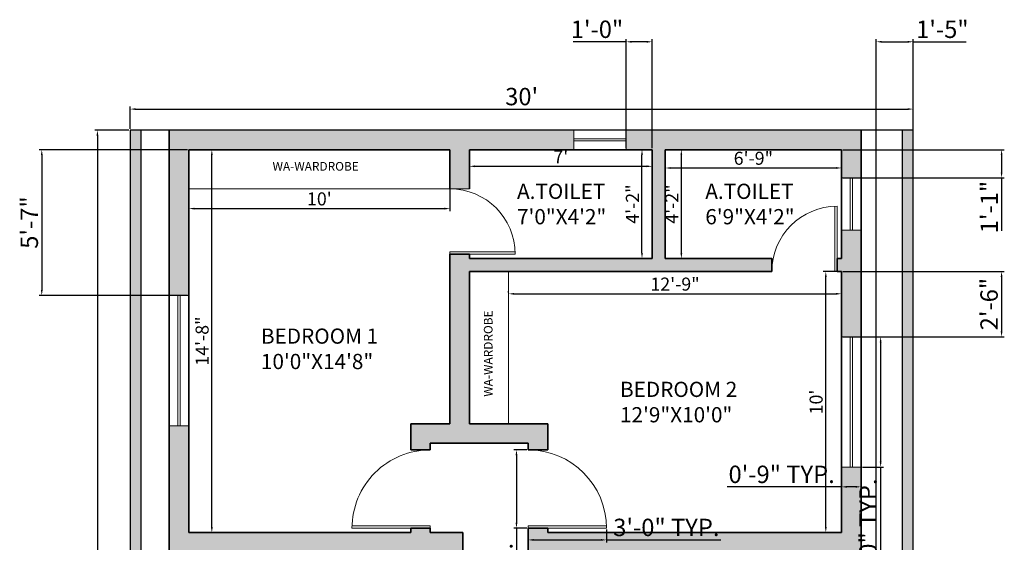
# Model space of a CAD drawing. Units: inches. Extents: x 2700 to 4052, y 1030 to 1872.
# Tile 8 of 8: x 3518 to 3971, y 1632 to 1872. Entities that reach past the tile are written whole.
import ezdxf

# ---------------------------------------------------------------- set-up
doc = ezdxf.new("R2010")
doc.units = ezdxf.units.IN
for name, color, linetype, lineweight in [('A-ANNO-DIMS', 2, 'Continuous', 13), ('A-ANNO-TEXT', 7, 'Continuous', 18), ('A-AREA-IDEN', 7, 'Continuous', 18), ('A-DOOR', 4, 'Continuous', 18), ('A-FLOR-CASE', 8, 'Continuous', 18), ('A-GLAZ', 4, 'Continuous', 18), ('A-WALL', 7, 'Continuous', 35), ('A-WALL-PATT', 7, 'Continuous', 13), ('C-PROP', 7, 'Continuous', 25)]:
    doc.layers.add(name, color=color, linetype=linetype, lineweight=lineweight)
doc.layers.add('C-SITE-PATT', color=252, linetype='Continuous', lineweight=13, true_color=0x939598)
doc.styles.get("Standard").update_dxf_attribs({"font": 'arial.ttf'})
doc.dimstyles.new('ISO-25', dxfattribs={"dimtxt": 8, "dimasz": 2.5, "dimexe": 1.25, "dimexo": 0.625, "dimtad": 1, "dimdec": 1, "dimlunit": 3, "dimtxsty": 'Standard', "dimcen": 2.5, "dimclrt": 1, "dimadec": 0, "dimazin": 0, "dimtfac": 1, "dimtdec": 1, "dimtmove": 0, "dimatfit": 3, "dimfxl": 1, "dimarcsym": 0})

# ---------------------------------------------------------------- blocks, each defined once
blk = doc.blocks.new('*D21')
at = {"layer": 'A-ANNO-DIMS', "color": 0, "lineweight": -2, "transparency": 16777216}
for p, q in [((3568.88, 1822.14), (3568.88, 1832.43)), ((3571.38, 1831.18), (3926.38, 1831.18)), ((3928.88, 1822.14), (3928.88, 1832.43))]:
    blk.add_line(p, q, dxfattribs=at)
at = {"layer": 'A-ANNO-DIMS', "color": 0, "transparency": 16777216}
for points in [[(3571.38, 1831.6), (3571.38, 1830.77), (3568.88, 1831.18)], [(3926.38, 1831.6), (3926.38, 1830.77), (3928.88, 1831.18)]]:
    blk.add_solid(points, dxfattribs=at)
at = {"layer": 'Defpoints', "color": 0, "transparency": 16777216}
for p in [(3928.88, 1831.18), (3568.88, 1821.52), (3928.88, 1821.52)]:
    blk.add_point(p, dxfattribs=at)
at = {"layer": 'A-ANNO-DIMS', "color": 0, "transparency": 16777216, "insert": (3748.88, 1835.89), "char_height": 8, "attachment_point": 5}
blk.add_mtext("30'", dxfattribs=at)
blk = doc.blocks.new('*D22')
at = {"layer": 'A-ANNO-DIMS', "color": 0, "lineweight": -2, "transparency": 16777216}
for p, q in [((3568.26, 1821.52), (3552.61, 1821.52)), ((3553.86, 1819.02), (3553.86, 1104.02)), ((3568.26, 1101.52), (3552.61, 1101.52))]:
    blk.add_line(p, q, dxfattribs=at)
at = {"layer": 'A-ANNO-DIMS', "color": 0, "transparency": 16777216}
for points in [[(3553.44, 1819.02), (3554.28, 1819.02), (3553.86, 1821.52)], [(3553.44, 1104.02), (3554.28, 1104.02), (3553.86, 1101.52)]]:
    blk.add_solid(points, dxfattribs=at)
at = {"layer": 'Defpoints', "color": 0, "transparency": 16777216}
for p in [(3568.88, 1821.52), (3553.86, 1101.52), (3568.88, 1101.52)]:
    blk.add_point(p, dxfattribs=at)
at = {"layer": 'A-ANNO-DIMS', "color": 0, "transparency": 16777216, "insert": (3549.15, 1461.52), "char_height": 8, "attachment_point": 5, "rotation": 90}
blk.add_mtext("60'", dxfattribs=at)
blk = doc.blocks.new('*D40')
at = {"layer": 'A-ANNO-DIMS', "color": 0, "lineweight": -2, "transparency": 16777216}
for p, q in [((3596.51, 1812.52), (3607.71, 1812.52)), ((3606.46, 1639.02), (3606.46, 1810.02)), ((3596.51, 1636.52), (3607.71, 1636.52))]:
    blk.add_line(p, q, dxfattribs=at)
at = {"layer": 'A-ANNO-DIMS', "color": 0, "transparency": 16777216}
for points in [[(3606.04, 1810.02), (3606.88, 1810.02), (3606.46, 1812.52)], [(3606.04, 1639.02), (3606.88, 1639.02), (3606.46, 1636.52)]]:
    blk.add_solid(points, dxfattribs=at)
at = {"layer": 'Defpoints', "color": 0, "transparency": 16777216}
for p in [(3595.88, 1812.52), (3606.46, 1812.52), (3595.88, 1636.52)]:
    blk.add_point(p, dxfattribs=at)
at = {"layer": 'A-ANNO-DIMS', "color": 0, "transparency": 16777216, "insert": (3602.77, 1724.52), "char_height": 6, "attachment_point": 5, "rotation": 90}
blk.add_mtext('14\'-8"', dxfattribs=at)
blk = doc.blocks.new('*D41')
at = {"layer": 'A-ANNO-DIMS', "color": 0, "lineweight": -2, "transparency": 16777216}
for p, q in [((3595.88, 1811.89), (3595.88, 1784.18)), ((3715.88, 1811.89), (3715.88, 1784.18)), ((3598.38, 1785.43), (3713.38, 1785.43))]:
    blk.add_line(p, q, dxfattribs=at)
at = {"layer": 'A-ANNO-DIMS', "color": 0, "transparency": 16777216}
for points in [[(3598.38, 1785.84), (3598.38, 1785.01), (3595.88, 1785.43)], [(3713.38, 1785.84), (3713.38, 1785.01), (3715.88, 1785.43)]]:
    blk.add_solid(points, dxfattribs=at)
at = {"layer": 'Defpoints', "color": 0, "transparency": 16777216}
for p in [(3595.88, 1812.52), (3715.88, 1812.52), (3715.88, 1785.43)]:
    blk.add_point(p, dxfattribs=at)
at = {"layer": 'A-ANNO-DIMS', "color": 0, "transparency": 16777216, "insert": (3655.88, 1789.12), "char_height": 6, "attachment_point": 5}
blk.add_mtext("10'", dxfattribs=at)
blk = doc.blocks.new('*D42')
at = {"layer": 'A-ANNO-DIMS', "color": 0, "lineweight": -2, "transparency": 16777216}
for p, q in [((3724.88, 1811.89), (3724.88, 1803.62)), ((3808.88, 1811.89), (3808.88, 1803.62)), ((3727.38, 1804.87), (3806.38, 1804.87))]:
    blk.add_line(p, q, dxfattribs=at)
at = {"layer": 'A-ANNO-DIMS', "color": 0, "transparency": 16777216}
for points in [[(3727.38, 1805.28), (3727.38, 1804.45), (3724.88, 1804.87)], [(3806.38, 1805.28), (3806.38, 1804.45), (3808.88, 1804.87)]]:
    blk.add_solid(points, dxfattribs=at)
at = {"layer": 'Defpoints', "color": 0, "transparency": 16777216}
for p in [(3724.88, 1812.52), (3808.88, 1812.52), (3808.88, 1804.87)]:
    blk.add_point(p, dxfattribs=at)
at = {"layer": 'A-ANNO-DIMS', "color": 0, "transparency": 16777216, "insert": (3766.88, 1808.49), "char_height": 6, "attachment_point": 5}
blk.add_mtext("7'", dxfattribs=at)
blk = doc.blocks.new('*D43')
at = {"layer": 'A-ANNO-DIMS', "color": 0, "lineweight": -2, "transparency": 16777216}
for p, q in [((3808.26, 1812.52), (3802.94, 1812.52)), ((3804.19, 1765.02), (3804.19, 1810.02)), ((3808.26, 1762.52), (3802.94, 1762.52))]:
    blk.add_line(p, q, dxfattribs=at)
at = {"layer": 'A-ANNO-DIMS', "color": 0, "transparency": 16777216}
for points in [[(3803.78, 1810.02), (3804.61, 1810.02), (3804.19, 1812.52)], [(3803.78, 1765.02), (3804.61, 1765.02), (3804.19, 1762.52)]]:
    blk.add_solid(points, dxfattribs=at)
at = {"layer": 'Defpoints', "color": 0, "transparency": 16777216}
for p in [(3804.19, 1812.52), (3808.88, 1812.52), (3808.88, 1762.52)]:
    blk.add_point(p, dxfattribs=at)
at = {"layer": 'A-ANNO-DIMS', "color": 0, "transparency": 16777216, "insert": (3800.56, 1787.52), "char_height": 6, "attachment_point": 5, "rotation": 90}
blk.add_mtext('4\'-2"', dxfattribs=at)
blk = doc.blocks.new('*D44')
at = {"layer": 'A-ANNO-DIMS', "color": 0, "lineweight": -2, "transparency": 16777216}
for p, q in [((3815.51, 1812.52), (3823.53, 1812.52)), ((3822.28, 1765.02), (3822.28, 1810.02)), ((3815.51, 1762.52), (3823.53, 1762.52))]:
    blk.add_line(p, q, dxfattribs=at)
at = {"layer": 'A-ANNO-DIMS', "color": 0, "transparency": 16777216}
for points in [[(3821.86, 1810.02), (3822.7, 1810.02), (3822.28, 1812.52)], [(3821.86, 1765.02), (3822.7, 1765.02), (3822.28, 1762.52)]]:
    blk.add_solid(points, dxfattribs=at)
at = {"layer": 'Defpoints', "color": 0, "transparency": 16777216}
for p in [(3814.88, 1812.52), (3822.28, 1812.52), (3814.88, 1762.52)]:
    blk.add_point(p, dxfattribs=at)
at = {"layer": 'A-ANNO-DIMS', "color": 0, "transparency": 16777216, "insert": (3818.64, 1787.52), "char_height": 6, "attachment_point": 5, "rotation": 90}
blk.add_mtext('4\'-2"', dxfattribs=at)
blk = doc.blocks.new('*D45')
at = {"layer": 'A-ANNO-DIMS', "color": 0, "lineweight": -2, "transparency": 16777216}
for p, q in [((3814.88, 1811.89), (3814.88, 1802.85)), ((3895.88, 1811.89), (3895.88, 1802.85)), ((3817.38, 1804.1), (3893.38, 1804.1))]:
    blk.add_line(p, q, dxfattribs=at)
at = {"layer": 'A-ANNO-DIMS', "color": 0, "transparency": 16777216}
for points in [[(3817.38, 1804.52), (3817.38, 1803.69), (3814.88, 1804.1)], [(3893.38, 1804.52), (3893.38, 1803.69), (3895.88, 1804.1)]]:
    blk.add_solid(points, dxfattribs=at)
at = {"layer": 'Defpoints', "color": 0, "transparency": 16777216}
for p in [(3814.88, 1812.52), (3895.88, 1812.52), (3895.88, 1804.1)]:
    blk.add_point(p, dxfattribs=at)
at = {"layer": 'A-ANNO-DIMS', "color": 0, "transparency": 16777216, "insert": (3855.38, 1807.79), "char_height": 6, "attachment_point": 5}
blk.add_mtext('6\'-9"', dxfattribs=at)
blk = doc.blocks.new('*D46')
at = {"layer": 'A-ANNO-DIMS', "color": 0, "lineweight": -2, "transparency": 16777216}
for p, q in [((3895.26, 1756.52), (3887.44, 1756.52)), ((3888.69, 1639.02), (3888.69, 1754.02)), ((3895.26, 1636.52), (3887.44, 1636.52))]:
    blk.add_line(p, q, dxfattribs=at)
at = {"layer": 'A-ANNO-DIMS', "color": 0, "transparency": 16777216}
for points in [[(3888.27, 1754.02), (3889.1, 1754.02), (3888.69, 1756.52)], [(3888.27, 1639.02), (3889.1, 1639.02), (3888.69, 1636.52)]]:
    blk.add_solid(points, dxfattribs=at)
at = {"layer": 'Defpoints', "color": 0, "transparency": 16777216}
for p in [(3888.69, 1756.52), (3895.88, 1756.52), (3895.88, 1636.52)]:
    blk.add_point(p, dxfattribs=at)
at = {"layer": 'A-ANNO-DIMS', "color": 0, "transparency": 16777216, "insert": (3885, 1696.52), "char_height": 6, "attachment_point": 5, "rotation": 90}
blk.add_mtext("10'", dxfattribs=at)
blk = doc.blocks.new('*D48')
at = {"layer": 'A-ANNO-DIMS', "color": 0, "lineweight": -2, "transparency": 16777216}
for p, q in [((3742.88, 1746.88), (3742.88, 1747.5)), ((3895.88, 1746.88), (3895.88, 1747.5)), ((3745.38, 1746.25), (3893.38, 1746.25))]:
    blk.add_line(p, q, dxfattribs=at)
at = {"layer": 'A-ANNO-DIMS', "color": 0, "transparency": 16777216}
for points in [[(3745.38, 1746.67), (3745.38, 1745.84), (3742.88, 1746.25)], [(3893.38, 1746.67), (3893.38, 1745.84), (3895.88, 1746.25)]]:
    blk.add_solid(points, dxfattribs=at)
at = {"layer": 'Defpoints', "color": 0, "transparency": 16777216}
for p in [(3742.88, 1746.25), (3895.88, 1746.25), (3895.88, 1746.25)]:
    blk.add_point(p, dxfattribs=at)
at = {"layer": 'A-ANNO-DIMS', "color": 0, "transparency": 16777216, "insert": (3819.38, 1749.94), "char_height": 6, "attachment_point": 5}
blk.add_mtext('12\'-9"', dxfattribs=at)
blk = doc.blocks.new('DOOR-SWING-36IN')
for p, q in [((-1, 36), (-1, 0)), ((0, 36), (0, 0)), ((0, 0), (-1, 0))]:
    blk.add_line(p, q)
blk.add_arc((0, 0), 36, 90, 180)
blk = doc.blocks.new('DOOR-SWING-30IN')
for p, q in [((-1, 30), (-1, 0)), ((0, 30), (0, 0)), ((0, 0), (-1, 0))]:
    blk.add_line(p, q)
blk.add_arc((0, 0), 30, 90, 180)
blk = doc.blocks.new('WINDOW-24IN')
for p, q in [((-4.5, 12), (4.5, 12)), ((-0.5, -12), (-0.5, 12)), ((0.5, -12), (0.5, 12)), ((-4.5, -12), (4.5, -12))]:
    blk.add_line(p, q)
blk = doc.blocks.new('WINDOW-60IN')
for p, q in [((4.5, 30), (-4.5, 30)), ((-0.5, 30), (-0.5, -30)), ((0.5, 30), (0.5, -30)), ((4.5, -30), (-4.5, -30))]:
    blk.add_line(p, q)
blk = doc.blocks.new('*D66')
at = {"layer": 'A-ANNO-DIMS', "color": 0, "lineweight": -2, "transparency": 16777216}
for p, q in [((3905.51, 1726.52), (3915.13, 1726.52)), ((3913.88, 1724.02), (3913.88, 1669.02)), ((3905.51, 1666.52), (3915.13, 1666.52)), ((3913.88, 1666.52), (3913.88, 1561.53))]:
    blk.add_line(p, q, dxfattribs=at)
at = {"layer": 'A-ANNO-DIMS', "color": 0, "transparency": 16777216}
for points in [[(3913.47, 1724.02), (3914.3, 1724.02), (3913.88, 1726.52)], [(3913.47, 1669.02), (3914.3, 1669.02), (3913.88, 1666.52)]]:
    blk.add_solid(points, dxfattribs=at)
at = {"layer": 'Defpoints', "color": 0, "transparency": 16777216}
for p in [(3904.88, 1726.52), (3904.88, 1666.52), (3913.88, 1666.52)]:
    blk.add_point(p, dxfattribs=at)
at = {"layer": 'A-ANNO-DIMS', "color": 1, "transparency": 16777216, "insert": (3909.12, 1612.78), "char_height": 8, "attachment_point": 5, "rotation": 90}
blk.add_mtext('WINDOW 5\'-0" TYP.', dxfattribs=at)
blk = doc.blocks.new('*D67')
at = {"layer": 'A-ANNO-DIMS', "color": 0, "lineweight": -2, "transparency": 16777216}
for p, q in [((3895.88, 1665.89), (3895.88, 1656.27)), ((3904.88, 1665.89), (3904.88, 1656.27)), ((3895.88, 1657.52), (3843.37, 1657.52)), ((3902.38, 1657.52), (3898.38, 1657.52))]:
    blk.add_line(p, q, dxfattribs=at)
at = {"layer": 'A-ANNO-DIMS', "color": 0, "transparency": 16777216}
for points in [[(3898.38, 1657.93), (3898.38, 1657.1), (3895.88, 1657.52)], [(3902.38, 1657.93), (3902.38, 1657.1), (3904.88, 1657.52)]]:
    blk.add_solid(points, dxfattribs=at)
at = {"layer": 'Defpoints', "color": 0, "transparency": 16777216}
for p in [(3895.88, 1666.52), (3904.88, 1666.52), (3895.88, 1657.52)]:
    blk.add_point(p, dxfattribs=at)
at = {"layer": 'A-ANNO-DIMS', "color": 1, "transparency": 16777216, "insert": (3868.38, 1662.23), "char_height": 8, "attachment_point": 5}
blk.add_mtext('0\'-9" TYP.', dxfattribs=at)
blk = doc.blocks.new('*D70')
at = {"layer": 'A-ANNO-DIMS', "color": 0, "lineweight": -2, "transparency": 16777216}
for p, q in [((3751.26, 1674.52), (3745.23, 1674.52)), ((3746.48, 1672.02), (3746.48, 1641.02)), ((3751.26, 1638.52), (3745.23, 1638.52)), ((3746.48, 1638.52), (3746.48, 1508.43))]:
    blk.add_line(p, q, dxfattribs=at)
at = {"layer": 'A-ANNO-DIMS', "color": 0, "transparency": 16777216}
for points in [[(3746.07, 1672.02), (3746.9, 1672.02), (3746.48, 1674.52)], [(3746.07, 1641.02), (3746.9, 1641.02), (3746.48, 1638.52)]]:
    blk.add_solid(points, dxfattribs=at)
at = {"layer": 'Defpoints', "color": 0, "transparency": 16777216}
for p in [(3751.88, 1674.52), (3746.48, 1638.52), (3751.88, 1638.52)]:
    blk.add_point(p, dxfattribs=at)
at = {"layer": 'A-ANNO-DIMS', "color": 1, "transparency": 16777216, "insert": (3741.72, 1572.22), "char_height": 8, "attachment_point": 5, "rotation": 90}
blk.add_mtext('SWING DOOR 3\'-0" TYP.', dxfattribs=at)
blk = doc.blocks.new('*D71')
at = {"layer": 'A-ANNO-DIMS', "color": 0, "lineweight": -2, "transparency": 16777216}
for p, q in [((3751.88, 1637.89), (3751.88, 1631.87)), ((3787.88, 1637.89), (3787.88, 1631.87)), ((3754.38, 1633.12), (3785.38, 1633.12)), ((3787.88, 1633.12), (3840.39, 1633.12))]:
    blk.add_line(p, q, dxfattribs=at)
at = {"layer": 'A-ANNO-DIMS', "color": 0, "transparency": 16777216}
for points in [[(3754.38, 1633.53), (3754.38, 1632.7), (3751.88, 1633.12)], [(3785.38, 1633.53), (3785.38, 1632.7), (3787.88, 1633.12)]]:
    blk.add_solid(points, dxfattribs=at)
at = {"layer": 'Defpoints', "color": 0, "transparency": 16777216}
for p in [(3751.88, 1638.52), (3787.88, 1638.52), (3787.88, 1633.12)]:
    blk.add_point(p, dxfattribs=at)
at = {"layer": 'A-ANNO-DIMS', "color": 1, "transparency": 16777216, "insert": (3815.39, 1637.83), "char_height": 8, "attachment_point": 5}
blk.add_mtext('3\'-0" TYP.', dxfattribs=at)
blk = doc.blocks.new('*D104')
at = {"layer": 'A-ANNO-DIMS', "color": 0, "lineweight": -2, "transparency": 16777216}
for p, q in [((3911.88, 1102.14), (3911.88, 1863.37)), ((3914.38, 1862.12), (3926.38, 1862.12)), ((3928.88, 1102.14), (3928.88, 1863.37)), ((3928.88, 1862.12), (3953.15, 1862.12))]:
    blk.add_line(p, q, dxfattribs=at)
at = {"layer": 'A-ANNO-DIMS', "color": 0, "transparency": 16777216}
for points in [[(3914.38, 1862.53), (3914.38, 1861.7), (3911.88, 1862.12)], [(3926.38, 1862.53), (3926.38, 1861.7), (3928.88, 1862.12)]]:
    blk.add_solid(points, dxfattribs=at)
at = {"layer": 'Defpoints', "color": 0, "transparency": 16777216}
for p in [(3928.88, 1862.12), (3911.88, 1101.52), (3928.88, 1101.52)]:
    blk.add_point(p, dxfattribs=at)
at = {"layer": 'A-ANNO-DIMS', "color": 1, "transparency": 16777216, "insert": (3942.26, 1866.83), "char_height": 8, "attachment_point": 5}
blk.add_mtext('1\'-5"', dxfattribs=at)
blk = doc.blocks.new('*D106')
at = {"layer": 'A-ANNO-DIMS', "color": 0, "lineweight": -2, "transparency": 16777216}
for p, q in [((3595.26, 1812.52), (3527.03, 1812.52)), ((3528.28, 1810.02), (3528.28, 1748.02)), ((3595.26, 1745.52), (3527.03, 1745.52))]:
    blk.add_line(p, q, dxfattribs=at)
at = {"layer": 'A-ANNO-DIMS', "color": 0, "transparency": 16777216}
for points in [[(3527.87, 1810.02), (3528.7, 1810.02), (3528.28, 1812.52)], [(3527.87, 1748.02), (3528.7, 1748.02), (3528.28, 1745.52)]]:
    blk.add_solid(points, dxfattribs=at)
at = {"layer": 'Defpoints', "color": 0, "transparency": 16777216}
for p in [(3595.88, 1812.52), (3528.28, 1745.52), (3595.88, 1745.52)]:
    blk.add_point(p, dxfattribs=at)
at = {"layer": 'A-ANNO-DIMS', "color": 1, "transparency": 16777216, "insert": (3523.59, 1779.02), "char_height": 8, "attachment_point": 5, "rotation": 90}
blk.add_mtext('5\'-7"', dxfattribs=at)
blk = doc.blocks.new('*D109')
at = {"layer": 'A-ANNO-DIMS', "color": 0, "lineweight": -2, "transparency": 16777216}
for p, q in [((3896.51, 1756.52), (3970.73, 1756.52)), ((3969.48, 1754.02), (3969.48, 1729.02)), ((3896.51, 1726.52), (3970.73, 1726.52))]:
    blk.add_line(p, q, dxfattribs=at)
at = {"layer": 'A-ANNO-DIMS', "color": 0, "transparency": 16777216}
for points in [[(3969.07, 1754.02), (3969.9, 1754.02), (3969.48, 1756.52)], [(3969.07, 1729.02), (3969.9, 1729.02), (3969.48, 1726.52)]]:
    blk.add_solid(points, dxfattribs=at)
at = {"layer": 'Defpoints', "color": 0, "transparency": 16777216}
for p in [(3895.88, 1756.52), (3895.88, 1726.52), (3969.48, 1726.52)]:
    blk.add_point(p, dxfattribs=at)
at = {"layer": 'A-ANNO-DIMS', "color": 1, "transparency": 16777216, "insert": (3964.77, 1741.52), "char_height": 8, "attachment_point": 5, "rotation": 90}
blk.add_mtext('2\'-6"', dxfattribs=at)
blk = doc.blocks.new('*D111')
at = {"layer": 'A-ANNO-DIMS', "color": 0, "lineweight": -2, "transparency": 16777216}
for p, q in [((3896.51, 1812.52), (3970.73, 1812.52)), ((3969.48, 1810.02), (3969.48, 1802.02)), ((3896.51, 1799.52), (3970.73, 1799.52)), ((3969.48, 1799.52), (3969.48, 1775.25))]:
    blk.add_line(p, q, dxfattribs=at)
at = {"layer": 'A-ANNO-DIMS', "color": 0, "transparency": 16777216}
for points in [[(3969.07, 1810.02), (3969.9, 1810.02), (3969.48, 1812.52)], [(3969.07, 1802.02), (3969.9, 1802.02), (3969.48, 1799.52)]]:
    blk.add_solid(points, dxfattribs=at)
at = {"layer": 'Defpoints', "color": 0, "transparency": 16777216}
for p in [(3895.88, 1812.52), (3895.88, 1799.52), (3969.48, 1799.52)]:
    blk.add_point(p, dxfattribs=at)
at = {"layer": 'A-ANNO-DIMS', "color": 1, "transparency": 16777216, "insert": (3964.84, 1786.14), "char_height": 8, "attachment_point": 5, "rotation": 90}
blk.add_mtext('1\'-1"', dxfattribs=at)
blk = doc.blocks.new('*D112')
at = {"layer": 'A-ANNO-DIMS', "color": 0, "lineweight": -2, "transparency": 16777216}
for p, q in [((3796.88, 1862.12), (3772.62, 1862.12)), ((3796.88, 1813.14), (3796.88, 1863.37)), ((3806.38, 1862.12), (3799.38, 1862.12)), ((3808.88, 1813.14), (3808.88, 1863.37))]:
    blk.add_line(p, q, dxfattribs=at)
at = {"layer": 'A-ANNO-DIMS', "color": 0, "transparency": 16777216}
for points in [[(3799.38, 1862.53), (3799.38, 1861.7), (3796.88, 1862.12)], [(3806.38, 1862.53), (3806.38, 1861.7), (3808.88, 1862.12)]]:
    blk.add_solid(points, dxfattribs=at)
at = {"layer": 'Defpoints', "color": 0, "transparency": 16777216}
for p in [(3796.88, 1862.12), (3796.88, 1812.52), (3808.88, 1812.52)]:
    blk.add_point(p, dxfattribs=at)
at = {"layer": 'A-ANNO-DIMS', "color": 1, "transparency": 16777216, "insert": (3783.5, 1866.83), "char_height": 8, "attachment_point": 5}
blk.add_mtext('1\'-0"', dxfattribs=at)

msp = doc.modelspace()

# ---------------------------------------------------------------- hatches: boundary and pattern name
at = {"layer": 'A-WALL-PATT'}
h = msp.add_hatch(color=256, dxfattribs=at)
h.dxf.hatch_style = 1
h.paths.add_polyline_path([(3904.88, 1539.52), (3895.88, 1539.52), (3895.88, 1479.52), (3904.88, 1479.52)])
h.paths.add_polyline_path([(3904.88, 1666.52), (3895.88, 1666.52), (3895.88, 1636.52), (3760.88, 1636.52), (3760.88, 1638.52), (3751.88, 1638.52), (3751.88, 1627.52), (3868.81, 1627.52, -0.035851), (3872.34, 1627.52), (3895.88, 1627.52), (3895.88, 1599.52), (3904.88, 1599.52)])
h.paths.add_polyline_path([(3595.88, 1537.52), (3586.88, 1537.52), (3586.88, 1486.52), (3595.88, 1486.52), (3595.88, 1501.52), (3677.88, 1501.52), (3677.88, 1507.52), (3595.88, 1507.52)], flags=17)
h.paths.add_polyline_path([(3595.88, 1438.52), (3586.88, 1438.52), (3586.88, 1423.52), (3568.88, 1423.52), (3568.88, 1414.52), (3616.88, 1414.52), (3616.88, 1412.52), (3625.88, 1412.52), (3625.88, 1423.52), (3595.88, 1423.52)])
h.paths.add_polyline_path([(3721.88, 1636.52), (3706.88, 1636.52), (3706.88, 1638.52), (3697.88, 1638.52), (3697.88, 1636.52), (3595.88, 1636.52), (3595.88, 1685.52), (3586.88, 1685.52), (3586.88, 1597.52), (3595.88, 1597.52), (3595.88, 1627.52), (3715.88, 1627.52), (3715.88, 1507.52), (3713.88, 1507.52), (3713.88, 1501.52), (3715.88, 1501.52), (3715.88, 1453.52), (3721.88, 1453.52)])
h.paths.add_polyline_path([(3724.88, 1756.52), (3863.88, 1756.52), (3863.88, 1762.52), (3814.88, 1762.52), (3814.88, 1812.52), (3895.88, 1812.52), (3895.88, 1799.52), (3904.88, 1799.52), (3904.88, 1821.52), (3796.88, 1821.52), (3796.88, 1812.52), (3808.88, 1812.52), (3808.88, 1762.52), (3724.88, 1762.52), (3724.88, 1764.52), (3715.88, 1764.52), (3715.88, 1686.52), (3697.88, 1686.52), (3697.88, 1674.52), (3706.88, 1674.52), (3706.88, 1677.52), (3751.88, 1677.52), (3751.88, 1674.52), (3760.88, 1674.52), (3760.88, 1686.52), (3724.88, 1686.52)])
h.paths.add_polyline_path([(3904.88, 1775.52), (3895.88, 1775.52), (3895.88, 1762.52), (3893.88, 1762.52), (3893.88, 1756.52), (3895.88, 1756.52), (3895.88, 1726.52), (3904.88, 1726.52)], flags=17)
h.paths.add_polyline_path([(3772.88, 1821.52), (3586.88, 1821.52), (3586.88, 1745.52), (3595.88, 1745.52), (3595.88, 1812.52), (3715.88, 1812.52), (3715.88, 1794.52), (3724.88, 1794.52), (3724.88, 1812.52), (3772.88, 1812.52)])
h = msp.add_hatch(color=256, dxfattribs=at)
h.dxf.hatch_style = 1
h.paths.add_polyline_path([(3651.88, 1264.52), (3625.88, 1264.52), (3625.88, 1310.49), (3616.88, 1310.49), (3616.88, 1304.37), (3616.88, 1264.52), (3568.88, 1264.52), (3568.88, 1168.52), (3709.88, 1168.52), (3709.88, 1177.52), (3577.88, 1177.52), (3577.88, 1255.52), (3651.88, 1255.52)])
h.paths.add_polyline_path([(3740.88, 1264.52), (3734.88, 1264.52), (3734.88, 1324.52), (3782.88, 1324.52), (3782.88, 1264.52), (3776.88, 1264.52), (3776.88, 1255.52), (3791.88, 1255.52), (3791.88, 1378.52), (3794.88, 1378.52), (3794.88, 1387.52), (3776.88, 1387.52), (3776.88, 1381.52), (3782.88, 1381.52), (3782.88, 1333.52), (3734.88, 1333.52), (3734.88, 1381.52), (3740.88, 1381.52), (3740.88, 1387.52), (3725.88, 1387.52), (3725.88, 1264.52), (3699.88, 1264.52), (3699.88, 1255.52), (3740.88, 1255.52)])
h.paths.add_polyline_path([(3625.88, 1382.52), (3616.88, 1382.52), (3616.88, 1358.49), (3625.88, 1358.49)])
h.paths.add_polyline_path([(3845.88, 1387.52), (3842.88, 1387.52), (3842.88, 1378.52), (3845.88, 1378.52)])
h.paths.add_polyline_path([(3904.88, 1431.52), (3895.88, 1431.52), (3895.88, 1387.52), (3893.88, 1387.52), (3893.88, 1378.52), (3895.88, 1378.52), (3895.88, 1300.52), (3904.88, 1300.52)])
h.paths.add_polyline_path([(3584.49, 1565.14), (3584.49, 1604.05), (3576.25, 1604.05), (3576.25, 1565.14)], flags=9)
h.paths.add_polyline_path([(3711.56, 1565.68), (3711.56, 1611.46), (3703.32, 1611.46), (3703.32, 1565.68)], flags=9)
h.paths.add_polyline_path([(3737.75, 1697.89), (3737.75, 1743.66), (3729.51, 1743.66), (3729.51, 1697.89)], flags=9)
h.paths.add_polyline_path([(3633.29, 1800.61), (3679.06, 1800.61), (3679.06, 1808.85), (3633.29, 1808.85)], flags=9)
h.paths.add_polyline_path([(3569.7, 1361.72), (3618.67, 1361.72), (3618.67, 1388.34), (3569.7, 1388.34)], flags=9)
h.paths.add_polyline_path([(3658.81, 1318.27), (3708.12, 1318.27), (3708.12, 1344.89), (3658.81, 1344.89)], flags=9)
h.paths.add_polyline_path([(3791.11, 1507.34), (3845.25, 1507.34), (3845.25, 1533.96), (3791.11, 1533.96)], flags=9)
h.paths.add_polyline_path([(3744.61, 1774.23), (3794.63, 1774.23), (3794.63, 1800.84), (3744.61, 1800.84)], flags=9)
h.paths.add_polyline_path([(3831.1, 1774.23), (3881.17, 1774.23), (3881.17, 1800.84), (3831.1, 1800.84)], flags=9)
h.paths.add_polyline_path([(3791.11, 1664.37), (3855.09, 1664.37), (3855.09, 1690.98), (3791.11, 1690.98)], flags=9)
h.paths.add_polyline_path([(3626.06, 1747.79), (3690.04, 1747.79), (3690.04, 1774.41), (3626.06, 1774.41)], flags=9)
h.paths.add_polyline_path([(3626.06, 1590.97), (3690.04, 1590.97), (3690.04, 1617.58), (3626.06, 1617.58)], flags=9)
h.paths.add_polyline_path([(3616.71, 1447.4), (3665.68, 1447.4), (3665.68, 1474.01), (3616.71, 1474.01)], flags=9)
at = {"layer": 'C-SITE-PATT'}
h = msp.add_hatch(color=256, dxfattribs=at)
h.dxf.hatch_style = 1
h.paths.add_polyline_path([(3573.88, 1821.52), (3568.88, 1821.52), (3568.88, 1423.52), (3573.88, 1423.52)])
h.paths.add_polyline_path([(3791.88, 1108.52), (3573.88, 1108.52), (3573.88, 1168.52), (3568.88, 1168.52), (3568.88, 1101.52), (3791.88, 1101.52)])
h.paths.add_polyline_path([(3928.88, 1821.52), (3923.88, 1821.52), (3923.88, 1108.52), (3911.88, 1108.52), (3911.88, 1101.52), (3928.88, 1101.52)])

# ---------------------------------------------------------------- linework, layer by layer
at = {"layer": 'A-FLOR-CASE'}
for p, q in [((3724.88, 1794.52), (3595.88, 1794.52)), ((3742.88, 1756.52), (3742.88, 1686.52))]:
    msp.add_line(p, q, dxfattribs=at)
at = {"layer": 'A-WALL'}
for p, q in [((3586.88, 1821.52), (3586.88, 1423.52)), ((3904.88, 1300.52), (3904.88, 1821.52)), ((3715.88, 1812.52), (3595.88, 1812.52)), ((3595.88, 1812.52), (3595.88, 1636.52)), ((3715.88, 1812.52), (3715.88, 1794.52)), ((3808.88, 1812.52), (3724.88, 1812.52)), ((3724.88, 1812.52), (3724.88, 1794.52)), ((3808.88, 1812.52), (3808.88, 1762.52)), ((3895.88, 1812.52), (3814.88, 1812.52)), ((3814.88, 1812.52), (3814.88, 1762.52)), ((3895.88, 1762.52), (3895.88, 1812.52)), ((3715.88, 1764.52), (3715.88, 1686.52)), ((3724.88, 1764.52), (3715.88, 1764.52)), ((3724.88, 1764.52), (3724.88, 1762.52)), ((3808.88, 1762.52), (3724.88, 1762.52)), ((3863.88, 1762.52), (3814.88, 1762.52)), ((3863.88, 1756.52), (3863.88, 1762.52)), ((3895.88, 1762.52), (3893.88, 1762.52)), ((3893.88, 1756.52), (3893.88, 1762.52)), ((3724.88, 1756.52), (3724.88, 1686.52)), ((3863.88, 1756.52), (3724.88, 1756.52)), ((3895.88, 1756.52), (3893.88, 1756.52)), ((3895.88, 1636.52), (3895.88, 1756.52)), ((3715.88, 1686.52), (3697.88, 1686.52)), ((3697.88, 1686.52), (3697.88, 1674.52)), ((3760.88, 1686.52), (3724.88, 1686.52)), ((3760.88, 1686.52), (3760.88, 1674.52)), ((3751.88, 1677.52), (3706.88, 1677.52)), ((3706.88, 1677.52), (3706.88, 1674.52)), ((3751.88, 1677.52), (3751.88, 1674.52)), ((3706.88, 1674.52), (3697.88, 1674.52)), ((3760.88, 1674.52), (3751.88, 1674.52)), ((3706.88, 1638.52), (3697.88, 1638.52)), ((3697.88, 1638.52), (3697.88, 1636.52)), ((3706.88, 1638.52), (3706.88, 1636.52)), ((3760.88, 1638.52), (3751.88, 1638.52)), ((3751.88, 1638.52), (3751.88, 1627.52)), ((3760.88, 1638.52), (3760.88, 1636.52)), ((3697.88, 1636.52), (3595.88, 1636.52)), ((3721.88, 1636.52), (3706.88, 1636.52)), ((3721.88, 1636.52), (3721.88, 1453.52)), ((3895.88, 1636.52), (3760.88, 1636.52))]:
    msp.add_line(p, q, dxfattribs=at)
at = {"layer": 'C-PROP'}
for p, q in [((3573.88, 1821.52), (3573.88, 1423.52)), ((3923.88, 1108.52), (3923.88, 1821.52))]:
    msp.add_line(p, q, dxfattribs=at)
msp.add_lwpolyline([(3911.88, 1101.52), (3928.88, 1101.52), (3928.88, 1821.52), (3568.88, 1821.52), (3568.88, 1101.52), (3791.88, 1101.52)], dxfattribs=at)

# ---------------------------------------------------------------- block references
at = {"layer": 'A-DOOR'}
for name, p, rotation in [('DOOR-SWING-30IN', (3715.88, 1764.52), 270.0000000000002), ('DOOR-SWING-36IN', (3751.88, 1638.52), 270.0000000000012)]:
    msp.add_blockref(name, p, dxfattribs=dict(at, rotation=rotation))
msp.add_blockref('DOOR-SWING-30IN', (3893.88, 1756.52), dxfattribs=at)
at = {"layer": 'A-DOOR', "extrusion": (0, 0, -1), "zscale": -1, "rotation": 270.0000000000019}
msp.add_blockref('DOOR-SWING-36IN', (-3706.88, 1638.52), dxfattribs=at)
at = {"layer": 'A-GLAZ'}
for name, p, rotation in [('WINDOW-24IN', (3784.88, 1817.02), 270.0000000000039), ('WINDOW-60IN', (3591.38, 1715.52), 180), ('WINDOW-60IN', (3900.38, 1696.52), 180)]:
    msp.add_blockref(name, p, dxfattribs=dict(at, rotation=rotation))
msp.add_blockref('WINDOW-24IN', (3900.38, 1787.52), dxfattribs=at)

# ---------------------------------------------------------------- texts
at = {"layer": 'A-ANNO-TEXT', "insert": (3634.36, 1806.86), "char_height": 4, "attachment_point": 1}
msp.add_mtext_dynamic_manual_height_columns('WA-WARDROBE', width=29.5334, gutter_width=12.5, heights=[0], dxfattribs=at)
at = {"layer": 'A-ANNO-TEXT', "insert": (3731.49, 1698.96), "char_height": 4, "attachment_point": 1, "rotation": 90}
msp.add_mtext_dynamic_manual_height_columns('WA-WARDROBE', width=29.5334, gutter_width=12.5, heights=[0], dxfattribs=at)
at = {"layer": 'A-AREA-IDEN', "char_height": 7, "attachment_point": 1}
for s, insert in [('{\\fTimes New Roman|b0|i0|c0|p18;A.TOILET\\P7\'0"X4\'2"}', (3746.75, 1796.88)), ('{\\fTimes New Roman|b0|i0|c0|p18;A.TOILET\\P6\'9"X4\'2"}', (3833.29, 1796.88)), ('{\\fTimes New Roman|b0|i0|c0|p18;BEDROOM 1\\P10\'0"X14\'8"}', (3629.02, 1730.31)), ('{\\fTimes New Roman|b0|i0|c0|p18;BEDROOM 2\\P12\'9"X10\'0"}', (3794.08, 1705.83))]:
    msp.add_mtext_dynamic_manual_height_columns(s, width=61.0557, gutter_width=12.5, heights=[0], dxfattribs=dict(at, insert=insert))

# ---------------------------------------------------------------- dimensions: what is measured, and where the dimension line sits
at = {"layer": 'A-ANNO-DIMS'}
for base, p1, p2, override, picture, middle in [((3796.88, 1862.12), (3808.88, 1812.52), (3796.88, 1812.52), {"dimdec": 1, "dimlfac": 1, "dimrnd": 0, "dimzin": 1, "dimdsep": 46, "dimlunit": 4, "dimfrac": 2}, '*D112', (3783.5, 1866.83)), ((3928.88, 1862.12), (3911.88, 1101.52), (3928.88, 1101.52), {"dimdec": 1, "dimlfac": 1, "dimrnd": 0, "dimzin": 1, "dimdsep": 46, "dimlunit": 4, "dimfrac": 2}, '*D104', (3942.26, 1866.83)), ((3928.88, 1831.18), (3568.88, 1821.52), (3928.88, 1821.52), {"dimclrd": 0, "dimclre": 0, "dimclrt": 0}, '*D21', (3748.88, 1835.89)), ((3715.88, 1785.43), (3595.88, 1812.52), (3715.88, 1812.52), {"dimtxt": 6, "dimclrd": 0, "dimclre": 0, "dimclrt": 0}, '*D41', (3655.88, 1789.12)), ((3808.88, 1804.87), (3724.88, 1812.52), (3808.88, 1812.52), {"dimtxt": 6, "dimclrd": 0, "dimclre": 0, "dimclrt": 0}, '*D42', (3766.88, 1808.49)), ((3895.88, 1804.1), (3814.88, 1812.52), (3895.88, 1812.52), {"dimtxt": 6, "dimclrd": 0, "dimclre": 0, "dimclrt": 0}, '*D45', (3855.38, 1807.79)), ((3895.88, 1746.25), (3742.88, 1746.25), (3895.88, 1746.25), {"dimtxt": 6, "dimclrd": 0, "dimclre": 0, "dimclrt": 0}, '*D48', (3819.38, 1749.94))]:
    dim = msp.add_linear_dim(base=base, p1=p1, p2=p2, dimstyle='ISO-25', override=override, dxfattribs=at)
    dim.commit()
    dim.dimension.update_dxf_attribs({"geometry": picture, "text_midpoint": middle})
for base, p1, p2, angle, override, picture, middle in [((3553.86, 1101.52), (3568.88, 1821.52), (3568.88, 1101.52), 90, {"dimclrd": 0, "dimclre": 0, "dimclrt": 0}, '*D22', (3549.15, 1461.52)), ((3528.28, 1745.52), (3595.88, 1812.52), (3595.88, 1745.52), 90, {"dimdec": 1, "dimlfac": 1, "dimrnd": 0, "dimzin": 1, "dimdsep": 46, "dimlunit": 4, "dimfrac": 2}, '*D106', (3523.59, 1779.02)), ((3606.46, 1812.52), (3595.88, 1636.52), (3595.88, 1812.52), 270, {"dimtxt": 6, "dimclrd": 0, "dimclre": 0, "dimclrt": 0}, '*D40', (3602.77, 1724.52)), ((3804.19, 1812.52), (3808.88, 1762.52), (3808.88, 1812.52), 270, {"dimtxt": 6, "dimclrd": 0, "dimclre": 0, "dimclrt": 0}, '*D43', (3800.56, 1787.52)), ((3822.28, 1812.52), (3814.88, 1762.52), (3814.88, 1812.52), 270, {"dimtxt": 6, "dimclrd": 0, "dimclre": 0, "dimclrt": 0}, '*D44', (3818.64, 1787.52)), ((3969.48, 1799.52), (3895.88, 1812.52), (3895.88, 1799.52), 90, {"dimdec": 1, "dimlfac": 1, "dimrnd": 0, "dimzin": 1, "dimdsep": 46, "dimlunit": 4, "dimfrac": 2}, '*D111', (3964.84, 1786.14)), ((3888.69, 1756.52), (3895.88, 1636.52), (3895.88, 1756.52), 270, {"dimtxt": 6, "dimclrd": 0, "dimclre": 0, "dimclrt": 0}, '*D46', (3885, 1696.52)), ((3969.48, 1726.52), (3895.88, 1756.52), (3895.88, 1726.52), 90, {"dimdec": 1, "dimlfac": 1, "dimrnd": 0, "dimzin": 1, "dimdsep": 46, "dimlunit": 4, "dimfrac": 2}, '*D109', (3964.77, 1741.52))]:
    dim = msp.add_linear_dim(base=base, p1=p1, p2=p2, angle=angle, dimstyle='ISO-25', override=override, dxfattribs=at)
    dim.commit()
    dim.dimension.update_dxf_attribs({"geometry": picture, "text_midpoint": middle})
for base, p1, p2, angle, text, picture, middle in [((3913.88, 1666.52), (3904.88, 1726.52), (3904.88, 1666.52), 270, 'WINDOW <> TYP.', '*D66', (3909.12, 1612.78)), ((3746.48, 1638.52), (3751.88, 1674.52), (3751.88, 1638.52), 270, 'SWING DOOR <> TYP.', '*D70', (3741.72, 1572.22)), ((3895.88, 1657.52), (3904.88, 1666.52), (3895.88, 1666.52), 180, '<> TYP.', '*D67', (3868.38, 1662.23)), ((3787.88, 1633.12), (3751.88, 1638.52), (3787.88, 1638.52), 0, '<> TYP.', '*D71', (3815.39, 1637.83))]:
    dim = msp.add_linear_dim(base=base, p1=p1, p2=p2, angle=angle, text=text, dimstyle='ISO-25', override={"dimdec": 1, "dimlfac": 1, "dimrnd": 0, "dimzin": 1, "dimdsep": 46, "dimlunit": 4, "dimfrac": 2}, dxfattribs=at)
    dim.commit()
    dim.dimension.update_dxf_attribs({"geometry": picture, "text_midpoint": middle})

doc.saveas('drawing.dxf')
